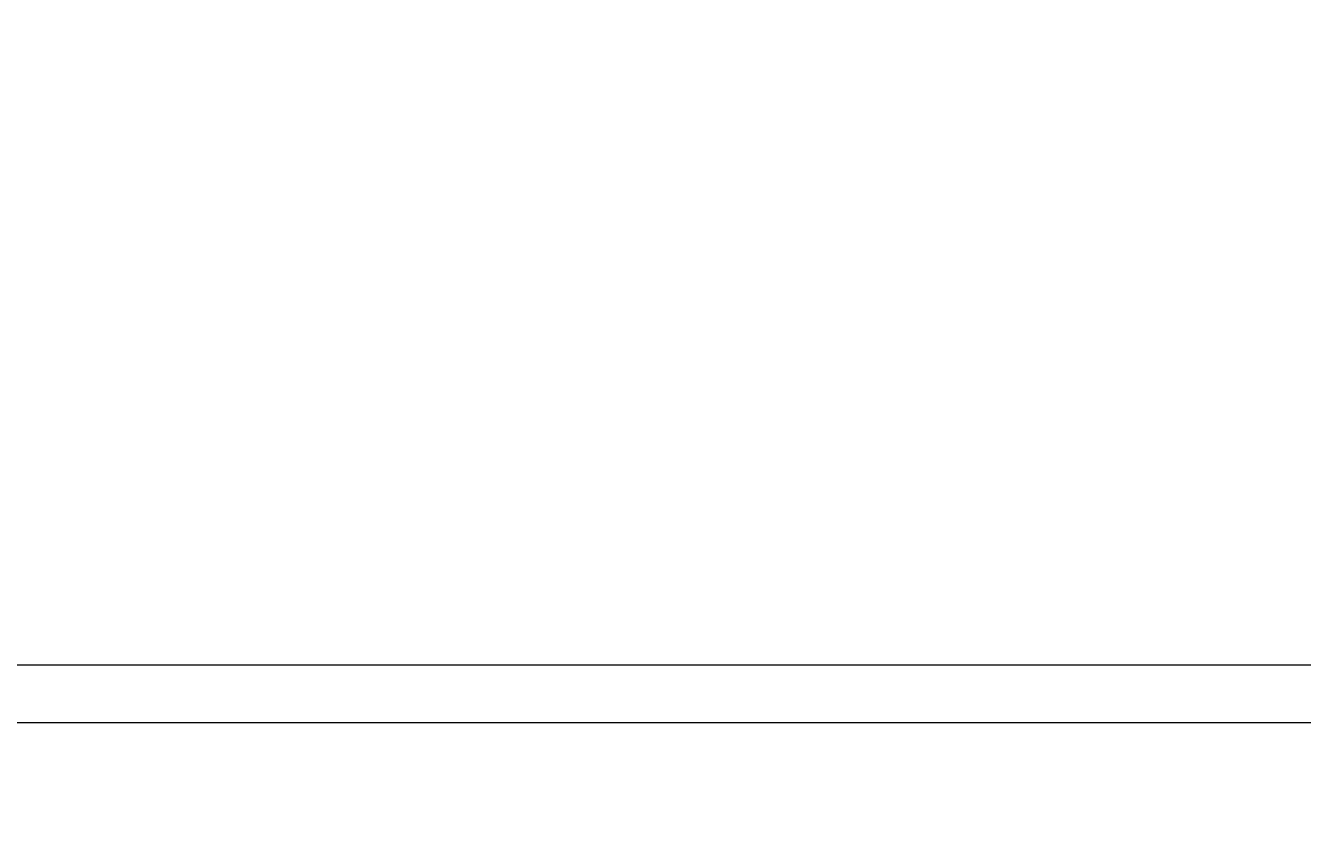
# Model space of a CAD drawing. Units: inches. Extents: x -61 to 1599, y -1316 to 257.
# Tile 116 of 204: x 109 to 134, y 11 to 27. Entities that reach past the tile are written whole.
import ezdxf

# ---------------------------------------------------------------- set-up
doc = ezdxf.new("R2010")
doc.units = ezdxf.units.IN
doc.header["$MEASUREMENT"] = 0
doc.layers.add('A-ANNO-DIMS', color=2, linetype='Continuous', lineweight=18)
doc.layers.add('FURNITURE', color=83, linetype='Continuous', lineweight=18)
doc.styles.get("Standard").update_dxf_attribs({"font": 'arial.ttf'})
doc.dimstyles.get("Standard").update_dxf_attribs({"dimtxt": 0.18, "dimasz": 0.18, "dimexe": 0.18, "dimexo": 0.0625, "dimgap": 0.09, "dimtad": 0, "dimtih": 1, "dimtoh": 1, "dimdec": 0, "dimzin": 0, "dimdsep": 46, "dimlunit": 3, "dimtxsty": 'Standard', "dimcen": 0.09, "dimadec": 0, "dimazin": 0, "dimtfac": 1, "dimtdec": 0, "dimtofl": 0, "dimtmove": 0, "dimatfit": 3, "dimfxl": 1, "dimtolj": 1, "dimtzin": 0, "dimarcsym": 0})

# ---------------------------------------------------------------- blocks, each defined once
blk = doc.blocks.new('BED-DOUBLE')
for p, q in [((1.272, 20.467), (70.263, 20.467)), ((1.272, 19.317), (70.263, 19.317))]:
    blk.add_line(p, q)
blk = doc.blocks.new('*D687')
at = {"layer": 'A-ANNO-DIMS', "color": 0, "lineweight": -2, "transparency": 16777216}
for p, q in [((289.418, 181.677), (-61.077, 181.677)), ((-60.897, 181.497), (-60.897, -528.952)), ((-60.897, -1239.765), (-60.897, -529.316)), ((319.64, -1239.945), (-61.077, -1239.945))]:
    blk.add_line(p, q, dxfattribs=at)
at = {"layer": 'A-ANNO-DIMS', "color": 0, "transparency": 16777216}
for points in [[(-60.927, 181.497), (-60.867, 181.497), (-60.897, 181.677)], [(-60.927, -1239.765), (-60.867, -1239.765), (-60.897, -1239.945)]]:
    blk.add_solid(points, dxfattribs=at)
at = {"layer": 'DEFPOINTS', "color": 0, "transparency": 16777216}
for p in [(289.481, 181.677), (-60.897, -1239.945), (319.703, -1239.945)]:
    blk.add_point(p, dxfattribs=at)
at = {"layer": 'A-ANNO-DIMS', "color": 0, "transparency": 16777216, "insert": (-60.897, -529.134), "char_height": 0.18, "attachment_point": 5}
blk.add_mtext('\\A1;1421.6', dxfattribs=at)
blk = doc.blocks.new('*D700')
at = {"layer": 'A-ANNO-DIMS', "color": 0, "lineweight": -2, "transparency": 16777216}
for p, q in [((14.703, -616.882), (14.703, 257.457)), ((179.752, -616.882), (179.752, 257.457)), ((14.883, 257.277), (96.772, 257.277)), ((179.572, 257.277), (97.683, 257.277))]:
    blk.add_line(p, q, dxfattribs=at)
at = {"layer": 'A-ANNO-DIMS', "color": 0, "transparency": 16777216}
for points in [[(14.883, 257.307), (14.883, 257.247), (14.703, 257.277)], [(179.572, 257.307), (179.572, 257.247), (179.752, 257.277)]]:
    blk.add_solid(points, dxfattribs=at)
at = {"layer": 'DEFPOINTS', "color": 0, "transparency": 16777216}
for p in [(179.752, 257.277), (14.703, -616.945), (179.752, -616.945)]:
    blk.add_point(p, dxfattribs=at)
at = {"layer": 'A-ANNO-DIMS', "color": 0, "transparency": 16777216, "insert": (97.227, 257.277), "char_height": 0.18, "attachment_point": 5}
blk.add_mtext('\\A1;165.05', dxfattribs=at)

msp = doc.modelspace()

# ---------------------------------------------------------------- block references
at = {"layer": 'FURNITURE'}
msp.add_blockref('BED-DOUBLE', (98.977, -5.797), dxfattribs=at)

# ---------------------------------------------------------------- dimensions: what is measured, and where the dimension line sits
at = {"layer": 'A-ANNO-DIMS'}
dim = msp.add_linear_dim(base=(179.7521, 257.2771), p1=(14.7028, -616.9446), p2=(179.7521, -616.9446), dimstyle='Standard', override={"dimdec": 2, "dimlfac": 1, "dimrnd": 0, "dimzin": 0, "dimdsep": 46, "dimlunit": 2}, dxfattribs=at)
dim.commit()
dim.dimension.update_dxf_attribs({"geometry": '*D700', "text_midpoint": (97.2274, 257.2771)})
dim = msp.add_linear_dim(base=(-60.8972, -1239.9446), p1=(289.4807, 181.6771), p2=(319.7028, -1239.9446), angle=90, dimstyle='Standard', override={"dimdec": 1, "dimlfac": 1, "dimrnd": 0, "dimzin": 0, "dimdsep": 46, "dimlunit": 2}, dxfattribs=at)
dim.commit()
dim.dimension.update_dxf_attribs({"geometry": '*D687', "text_midpoint": (-60.8972, -529.1337)})

doc.saveas('drawing.dxf')
